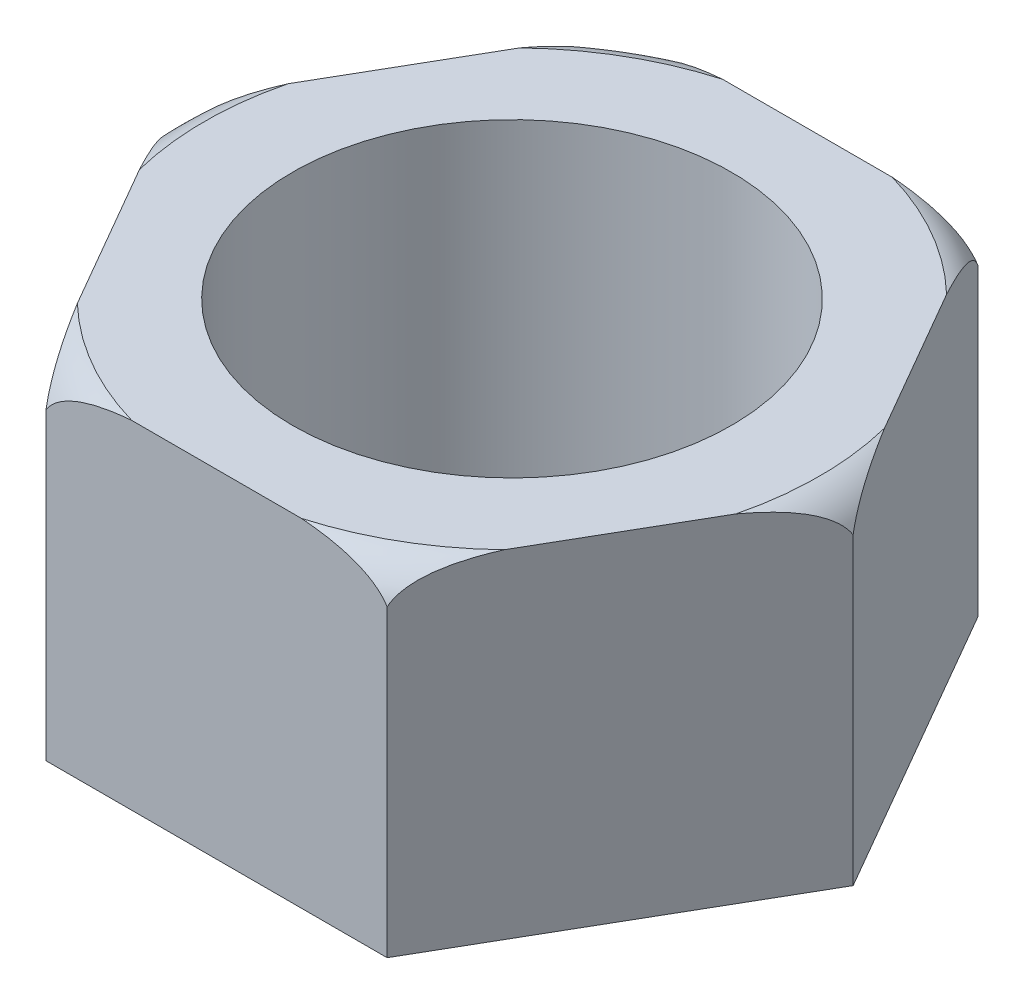
SolidWorks part; units mm, degrees
material "Plain Carbon Steel"
ref_plane "Front Plane" through (0, 0, 0) normal (0, 0, 1) x (1, 0, 0)
ref_plane "Top Plane" through (0, 0, 0) normal (0, 1, 0) x (1, 0, 0)
ref_plane "Right Plane" through (0, 0, 0) normal (1, 0, 0) x (0, 0, -1)
sketch "Hex Profile Sketch" plane through (0, 0, 0) normal (0, 1, 0) x (1, 0, 0)
  line L1 (20.2073, 0) -> (10.1036, 17.5)
  line L2 (10.1036, 17.5) -> (-10.1036, 17.5)
  line L3 (-10.1036, 17.5) -> (-20.2073, 0)
  line L4 (-20.2073, 0) -> (-10.1036, -17.5)
  line L5 (-10.1036, -17.5) -> (10.1036, -17.5)
  line L6 (10.1036, -17.5) -> (20.2073, 0)
  circle A0 centre (0, 0) radius 17.5 construction
  circle A1 centre (0, 0) radius 13
  dimension "D1" = 26
  dimension "D2" = 35
extrude "Hex Nut Body" add sketch "Hex Profile Sketch" along normal mid plane 20
sketch "Corner Chamfer Profile" plane through (0, 0, 0) normal (0, 0, 1) x (1, 0, 0)
  line L0 (10.1036, 10) -> (20.2073, 10) construction
  line L1 (20.2073, 10) -> (20.2073, -10) construction
  line L2 (18.2073, 10) -> (20.2073, 10)
  line L3 (20.2073, 10) -> (20.2073, 8)
  line L4 (0, 0) -> (0, 18.6733) construction
  arc A0 (18.2073, 10) -> (20.2073, 8) centre (17.3364, 7.1292) cw
  dimension "D3" = 3
  dimension "D1" = 2
  dimension "D2" = 2
revolve "Corner Chamfer Cut" cut sketch "Corner Chamfer Profile" angle 360 about L4
